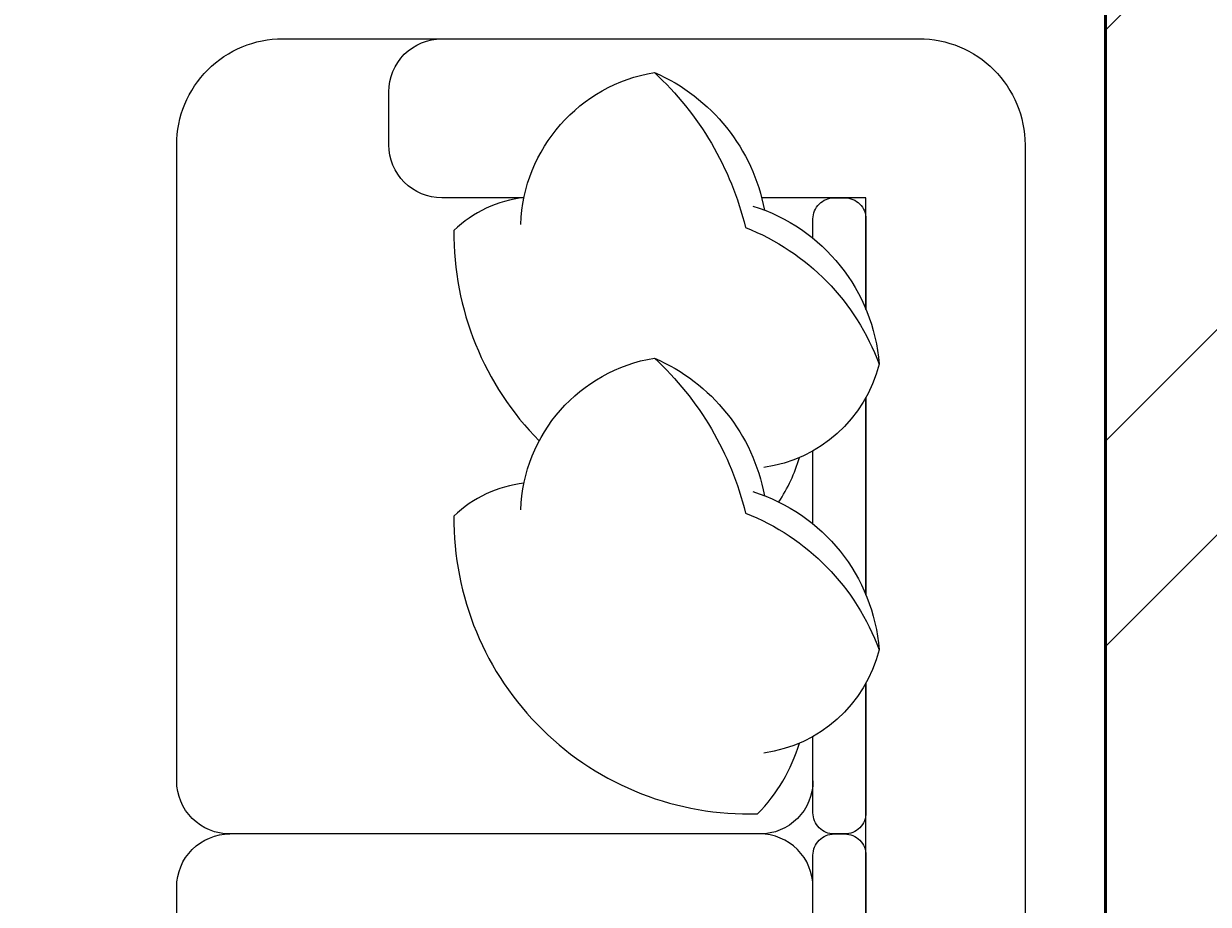
# Model space of a CAD drawing. Units: inches. Extents: x 963 to 2075, y 289 to 2657.
# Tile 24 of 98: x 1485 to 1511, y 1781 to 1800. Entities that reach past the tile are written whole.
import ezdxf

# ---------------------------------------------------------------- set-up
doc = ezdxf.new("R2010")
doc.units = ezdxf.units.IN
for name, color, linetype, lineweight in [('A-ANNO-DIMS', 2, 'Continuous', 18), ('A-FURN', 8, 'Continuous', 18), ('A-WALL', 7, 'Continuous', 50), ('A-WALL-PATT', 8, 'Continuous', 13)]:
    doc.layers.add(name, color=color, linetype=linetype, lineweight=lineweight)
doc.styles.get("Standard").update_dxf_attribs({"font": 'arial.ttf'})
doc.dimstyles.get("Standard").update_dxf_attribs({"dimtxt": 0.18, "dimasz": 0.18, "dimexe": 0.18, "dimexo": 0.0625, "dimgap": 0.09, "dimtad": 0, "dimtih": 1, "dimtoh": 1, "dimdec": 4, "dimzin": 0, "dimdsep": 46, "dimtxsty": 'Standard', "dimcen": 0.09, "dimadec": 0, "dimazin": 0, "dimtfac": 1, "dimtdec": 4, "dimtofl": 0, "dimtmove": 0, "dimatfit": 3, "dimfxl": 1, "dimtolj": 1, "dimtzin": 0, "dimarcsym": 0})

# ---------------------------------------------------------------- blocks, each defined once
blk = doc.blocks.new('SOFA-3SEAT')
at = {"ltscale": 0.03}
blk.add_lwpolyline([(2.442, 16.426, -0.414214), (0.124, 18.743), (0.124, 32.649, -0.414214), (1.283, 33.808, -0.414214), (0.124, 34.967), (0.124, 46.555, -0.414214), (1.283, 47.713, -0.414214), (0.124, 48.872), (0.124, 62.778, -0.414214), (2.442, 65.095), (16.347, 65.095, -0.414214), (18.665, 62.778), (18.665, 18.743, -0.414214), (16.347, 16.426)], format="xyb", close=True, dxfattribs=at)
for points in [[(7.713, 61.619), (5.918, 61.619, -0.414214), (4.759, 62.778), (4.759, 63.937, -0.414214), (5.918, 65.095)], [(7.643, 61.038, -0.356772), (10.564, 64.358, -0.249542), (12.971, 61.349, 9.61688)], [(10.564, 64.358, -0.14773), (12.556, 60.971, -0.213343), (15.477, 57.983, -0.178662)], [(7.714, 61.622, 0.165541), (6.183, 60.905, 0.200231), (8.048, 56.305, 0.121523)], [(12.714, 61.439, -0.306663), (15.477, 57.983, -0.30633), (12.954, 55.725, 0.872847)], [(15.189, 59.181), (15.189, 61.619), (12.911, 61.619, -0.414214)], [(14.03, 60.735), (14.03, 61.156, -0.414214), (14.493, 61.619), (14.725, 61.619, -0.414214), (15.189, 61.156)], [(15.189, 61.156), (15.189, 59.181, -0.414214)], [(7.643, 54.795, -0.356772), (10.564, 58.116, -0.249542), (12.971, 55.107, 9.61688)], [(10.564, 58.116, -0.14773), (12.556, 54.729, -0.213343), (15.477, 51.74, -0.178662)], [(15.189, 57.253), (15.189, 52.939, -0.414214)], [(13.283, 54.97, 0.071865), (13.736, 55.942, -7.115464)], [(14.03, 54.492), (14.03, 56.087, -0.414214)], [(7.714, 55.379, 0.165541), (6.183, 54.662, 0.425989), (12.821, 48.154, 0.121523), (13.736, 49.699, -7.115464)], [(12.714, 55.197, -0.306663), (15.477, 51.74, -0.30633), (12.954, 49.482, 0.872847)], [(15.189, 51.011), (15.189, 48.177, -0.414214), (14.725, 47.713), (14.493, 47.713, -0.414214), (14.03, 48.177), (14.03, 49.844, -0.414214)], [(14.03, 48.872, -0.414214), (12.871, 47.713), (1.283, 47.713, -0.414214)], [(14.03, 46.555, 0.414214), (12.871, 47.713)]]:
    blk.add_lwpolyline(points, format="xyb")
for points in [[(15.189, 52.939), (15.189, 57.253)], [(15.189, 24.268), (15.189, 51.011)]]:
    blk.add_lwpolyline(points)
blk.add_lwpolyline([(15.189, 47.25), (15.189, 34.271, -0.414214), (14.725, 33.808), (14.493, 33.808, -0.414214), (14.03, 34.271), (14.03, 47.25, -0.414214), (14.493, 47.713), (14.725, 47.713, -0.414214)], format="xyb", close=True)
blk = doc.blocks.new('*D28')
at = {"layer": 'A-ANNO-DIMS', "color": 0, "lineweight": -2, "transparency": 16777216}
for p, q in [((1506.727, 1816.319), (1519.012, 1816.319)), ((1518.832, 1816.139), (1518.832, 1775.944)), ((1518.832, 1735.382), (1518.832, 1775.577)), ((1506.727, 1735.202), (1519.012, 1735.202))]:
    blk.add_line(p, q, dxfattribs=at)
at = {"layer": 'A-ANNO-DIMS', "color": 0, "transparency": 16777216}
for points in [[(1518.802, 1816.139), (1518.862, 1816.139), (1518.832, 1816.319)], [(1518.802, 1735.382), (1518.862, 1735.382), (1518.832, 1735.202)]]:
    blk.add_solid(points, dxfattribs=at)
at = {"layer": 'Defpoints', "color": 0, "transparency": 16777216}
for p in [(1506.665, 1816.319), (1518.832, 1816.319), (1506.665, 1735.202)]:
    blk.add_point(p, dxfattribs=at)
at = {"layer": 'A-ANNO-DIMS', "color": 0, "transparency": 16777216, "insert": (1518.832, 1775.761), "char_height": 0.18, "attachment_point": 5}
blk.add_mtext('\\A1;3-SEAT SOFA 81 TYP.', dxfattribs=at)

msp = doc.modelspace()

# ---------------------------------------------------------------- hatches: boundary and pattern name
at = {"layer": 'A-WALL-PATT'}
h = msp.add_hatch(dxfattribs=at)
h.set_pattern_fill('ANSI32', color=256)
h.paths.add_polyline_path([(1473.609, 2163.068), (1473.609, 2165.318), (1376.422, 2165.318), (1376.422, 2227.983), (1371.922, 2227.983), (1371.922, 2214.818), (1368.405, 2214.818), (1368.405, 2210.318), (1371.922, 2210.318), (1371.922, 2160.818), (1395.922, 2160.818), (1395.922, 2090.318), (1217.345, 2090.318), (1217.345, 2085.818), (1395.922, 2085.818), (1458.922, 2085.818), (1458.922, 2108.318), (1454.422, 2108.318), (1454.422, 2090.318), (1400.422, 2090.318), (1400.422, 2160.818), (1473.609, 2160.818)])
h.paths.add_polyline_path([(1649.422, 2210.318), (1653.225, 2210.318), (1653.225, 2214.818), (1649.422, 2214.818), (1649.422, 2227.983), (1644.922, 2227.983), (1644.922, 2165.318), (1550.099, 2165.318), (1550.099, 2160.818), (1620.922, 2160.818), (1620.922, 2112.818), (1555.446, 2112.818), (1555.446, 2108.318), (1584.327, 2108.318), (1584.327, 2084.916), (1588.827, 2084.916), (1588.827, 2108.318), (1625.422, 2108.318), (1667.951, 2108.318), (1667.951, 2022.667), (1588.827, 2022.667), (1588.827, 2047.408), (1584.327, 2047.408), (1584.327, 1996.003), (1588.827, 1996.003), (1588.827, 2018.318), (1667.951, 2018.167), (1667.951, 1928.318), (1625.422, 1928.318), (1625.422, 1923.818), (1672.451, 1923.818), (1672.451, 1928.318), (1672.451, 1946.663), (1785.446, 1946.663), (1785.446, 1951.163), (1743.034, 1951.163), (1743.034, 2017.922), (1841.422, 2017.922), (1841.422, 2014.775), (1845.922, 2014.775), (1845.922, 2017.922), (1905.922, 2017.922), (1905.922, 1987.511), (1910.422, 1987.511), (1910.422, 2022.422), (1910.422, 2068.517), (1905.922, 2068.517), (1905.922, 2022.422), (1845.922, 2022.422), (1845.922, 2025.851), (1843.672, 2025.851), (1841.422, 2025.851), (1841.422, 2022.422), (1743.034, 2022.422), (1743.034, 2084.031), (1768.451, 2084.031), (1785.446, 2084.031), (1785.446, 2088.531), (1672.451, 2088.531), (1672.451, 2112.818), (1667.951, 2112.818), (1625.422, 2112.818), (1625.422, 2160.818), (1649.422, 2160.818)])
h.paths.add_polyline_path([(1672.451, 2084.031), (1738.534, 2084.031), (1738.534, 1951.163), (1672.451, 1951.163)], flags=16)
h.paths.add_polyline_path([(1672.451, 2084.031), (1738.534, 2084.031), (1705.492, 2017.597)], flags=0)
h.paths.add_polyline_path([(1262.766, 2085.818), (1258.266, 2085.818), (1258.266, 2023.278), (1184.422, 2023.278), (1184.422, 2018.778), (1258.266, 2018.778), (1258.266, 1950.818), (1262.766, 1950.818)])
h.paths.add_polyline_path([(1312.266, 2085.818), (1307.766, 2085.818), (1307.766, 1950.818), (1312.266, 1950.818)])
h.paths.add_polyline_path([(1458.922, 1950.818), (1395.922, 1950.818), (1216.568, 1950.818), (1216.568, 1946.318), (1346.422, 1946.318), (1395.922, 1946.318), (1395.922, 1875.818), (1371.922, 1875.818), (1371.922, 1826.318), (1368.931, 1826.318), (1368.931, 1821.818), (1371.922, 1821.818), (1371.922, 1813.622), (1376.422, 1813.622), (1376.422, 1871.318), (1474.504, 1871.318), (1474.504, 1873.568), (1474.504, 1875.818), (1400.422, 1875.818), (1400.422, 1946.318), (1454.422, 1946.318), (1454.422, 1928.318), (1458.922, 1928.318)])
h.paths.add_polyline_path([(1184.422, 2120.778), (1167.922, 2120.778), (1167.922, 2134.812), (1165.672, 2134.812), (1163.422, 2134.812), (1163.422, 2120.778), (1119.922, 2120.778), (1119.922, 2098.095), (1124.422, 2098.095), (1124.422, 2116.278), (1167.922, 2116.278), (1179.922, 2116.278), (1179.922, 2045.916), (1184.422, 2045.916), (1184.422, 2090.318), (1184.422, 2116.278)])
h.paths.add_polyline_path([(1124.422, 2018.778), (1179.922, 2018.778), (1179.922, 2016.294), (1184.422, 2016.294), (1184.422, 2023.278), (1184.422, 2026.588), (1182.172, 2026.588), (1179.922, 2026.588), (1179.922, 2023.278), (1124.422, 2023.278), (1124.422, 2074.095), (1119.922, 2074.095), (1119.922, 2018.778), (1119.922, 1979.633), (1124.422, 1979.633)])
h.paths.add_polyline_path([(1184.422, 1925.778), (1184.422, 1946.318), (1184.422, 1996.073), (1182.172, 1996.073), (1179.922, 1996.073), (1179.922, 1925.778), (1124.422, 1925.778), (1124.422, 1955.633), (1119.922, 1955.502), (1119.922, 1921.278), (1158.922, 1921.278), (1158.922, 1909.983), (1163.422, 1909.983), (1163.422, 1921.278), (1184.422, 1921.278)])
h.paths.add_polyline_path([(1341.449, 1826.318), (1163.422, 1826.318), (1163.422, 1849.983), (1158.922, 1849.983), (1158.922, 1821.818), (1158.922, 1804.033), (1163.422, 1804.033), (1163.422, 1821.818), (1341.449, 1821.818)])
h.paths.add_polyline_path([(1222.981, 1713.818), (1163.422, 1713.818), (1163.422, 1744.033), (1161.172, 1744.033), (1158.922, 1744.033), (1158.922, 1713.818), (1119.922, 1713.818), (1119.922, 1694.65), (1124.422, 1694.65), (1124.422, 1709.318), (1158.922, 1709.318), (1222.981, 1709.318)])
h.paths.add_polyline_path([(1328.422, 1713.818), (1252.042, 1713.818), (1252.042, 1711.568), (1252.042, 1709.318), (1256.422, 1709.318), (1256.422, 1547.318), (1232.937, 1547.318), (1232.937, 1545.068), (1232.937, 1542.818), (1292.422, 1542.818), (1292.422, 1527.634), (1296.922, 1527.634), (1296.922, 1542.818), (1299.464, 1542.818), (1299.464, 1547.318), (1260.922, 1547.318), (1260.922, 1658.318), (1343.661, 1658.318), (1343.661, 1660.568), (1343.661, 1662.818), (1328.422, 1662.818), (1328.422, 1676.589), (1327.402, 1676.589), (1323.922, 1676.589), (1323.922, 1662.818), (1260.922, 1662.818), (1260.922, 1709.318), (1323.922, 1709.318), (1323.922, 1699.851), (1328.422, 1699.851)])
h.paths.add_polyline_path([(1649.422, 1875.818), (1625.422, 1875.818), (1625.422, 1928.318), (1620.922, 1928.318), (1588.827, 1928.318), (1588.827, 1950.59), (1584.327, 1950.59), (1584.327, 1928.318), (1555.446, 1928.318), (1555.446, 1923.818), (1620.922, 1923.818), (1620.922, 1875.818), (1548.952, 1875.818), (1548.952, 1873.568), (1548.952, 1871.318), (1644.922, 1871.318), (1644.922, 1813.622), (1649.422, 1813.622), (1649.422, 1821.818), (1652.045, 1821.818), (1652.045, 1824.068), (1652.045, 1826.318), (1649.422, 1826.318)])
h.paths.add_polyline_path([(1512.922, 1871.318), (1516.476, 1871.318), (1516.476, 1875.818), (1512.922, 1875.818), (1512.922, 1923.818), (1512.922, 1928.318), (1512.922, 1930.827), (1508.422, 1930.827), (1508.422, 1875.818), (1504.411, 1875.818), (1504.411, 1871.318), (1508.422, 1871.318), (1508.422, 1713.818), (1376.422, 1713.818), (1376.422, 1743.325), (1371.922, 1743.325), (1371.922, 1709.318), (1371.922, 1706.01), (1376.422, 1706.01), (1376.422, 1709.318), (1508.422, 1709.318), (1508.422, 1547.318), (1501.871, 1547.318), (1501.871, 1542.818), (1508.422, 1542.818), (1508.422, 1482.818), (1508.422, 1436.318), (1512.922, 1436.318), (1512.922, 1542.818), (1519.318, 1542.818), (1519.318, 1545.068), (1519.318, 1547.318), (1512.922, 1547.318), (1512.922, 1709.318), (1644.922, 1709.318), (1644.922, 1707.548), (1649.422, 1707.548), (1649.422, 1709.318), (1649.422, 1743.325), (1644.922, 1743.325), (1644.922, 1713.818), (1512.922, 1713.818)])
h.paths.add_polyline_path([(1129.884, 1545.068), (1129.884, 1547.318), (1124.422, 1547.318), (1095.922, 1547.318), (1095.922, 1614.818), (1124.422, 1614.818), (1124.422, 1619.318), (1095.922, 1619.318), (1091.422, 1619.318), (1091.422, 1542.818), (1095.922, 1542.818), (1119.922, 1542.818), (1129.884, 1542.818)])
h.paths.add_polyline_path([(1208.422, 1542.818), (1211.74, 1542.818), (1211.74, 1547.318), (1198.851, 1547.318), (1198.851, 1542.818), (1203.922, 1542.818), (1203.922, 1478.318), (1208.422, 1478.318), (1296.922, 1478.318), (1296.922, 1503.634), (1292.422, 1503.634), (1292.422, 1482.818), (1208.422, 1482.818)])
h.paths.add_polyline_path([(1430.422, 1542.818), (1435.699, 1542.818), (1435.699, 1545.068), (1435.699, 1547.318), (1422.658, 1547.318), (1422.658, 1545.068), (1422.658, 1542.818), (1425.922, 1542.818), (1425.922, 1482.857), (1341.922, 1482.857), (1341.922, 1502.732), (1337.422, 1502.732), (1337.422, 1478.357), (1425.922, 1478.357), (1425.922, 1440.818), (1425.922, 1436.318), (1430.422, 1436.318)])
h.paths.add_polyline_path([(1698.482, 2004.259), (1727.695, 2004.259), (1727.695, 2022.916), (1698.482, 2022.916)], flags=8)

# ---------------------------------------------------------------- linework, layer by layer
at = {"layer": 'A-WALL'}
msp.add_line((1508.422, 1871.318), (1508.422, 1713.818), dxfattribs=at)

# ---------------------------------------------------------------- block references
at = {"layer": 'A-FURN'}
msp.add_blockref('SOFA-3SEAT', (1488, 1735), dxfattribs=at)

# ---------------------------------------------------------------- dimensions: what is measured, and where the dimension line sits
at = {"layer": 'A-ANNO-DIMS'}
dim = msp.add_linear_dim(base=(1518.832, 1816.319), p1=(1506.665, 1735.202), p2=(1506.665, 1816.319), angle=90, text='3-SEAT SOFA <> TYP.', dimstyle='Standard', override={"dimdec": 0, "dimlfac": 1, "dimrnd": 0, "dimzin": 0, "dimdsep": 46, "dimlunit": 2}, dxfattribs=at)
dim.commit()
dim.dimension.update_dxf_attribs({"geometry": '*D28', "text_midpoint": (1518.832, 1775.761)})

doc.saveas('drawing.dxf')
